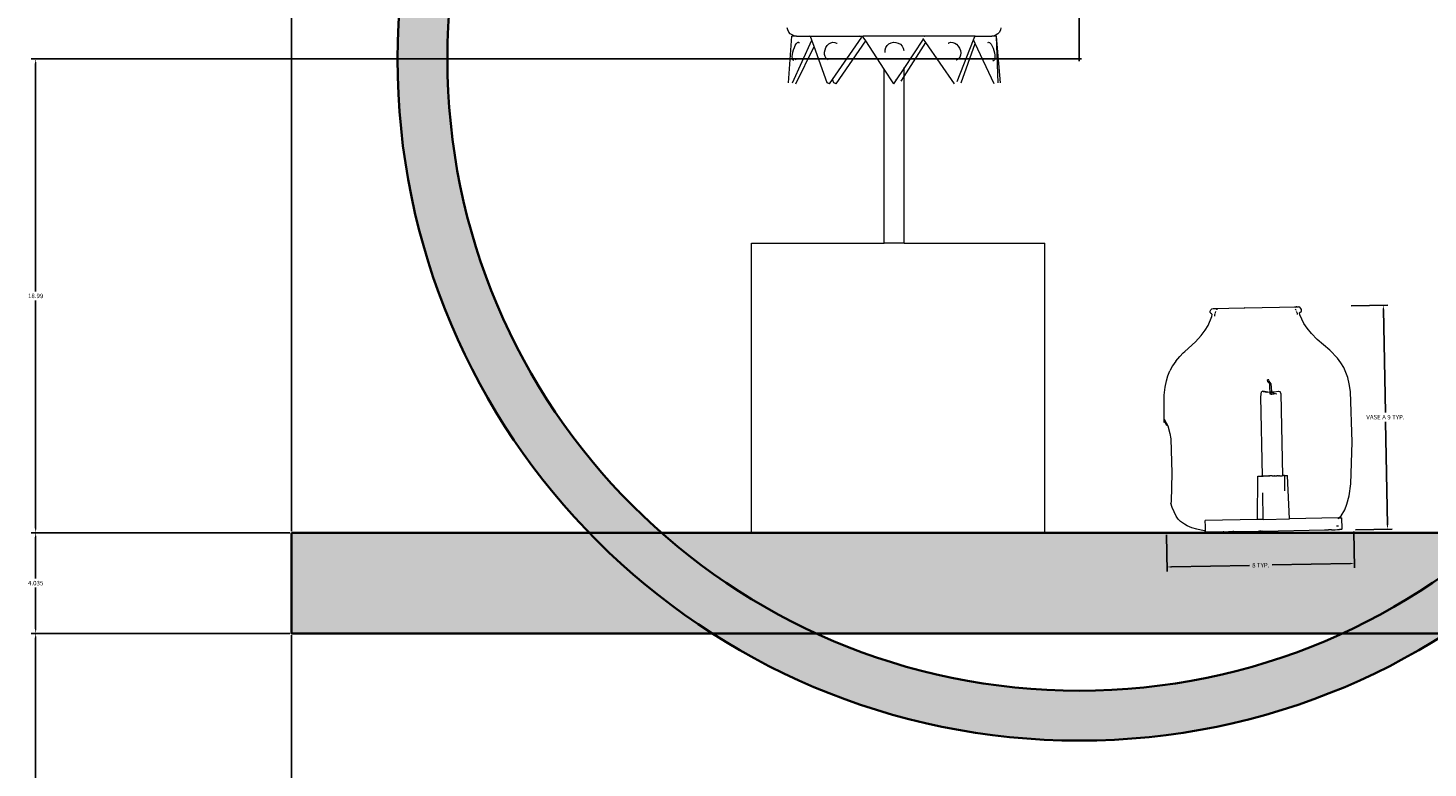
# Model space of a CAD drawing. Units: millimetres. Extents: x 446512 to 447461, y 70395 to 70610.
# Tile 29 of 39: x 447244 to 447300, y 70447 to 70477. Entities that reach past the tile are written whole.
import ezdxf

# ---------------------------------------------------------------- set-up
doc = ezdxf.new("R2010")
doc.units = ezdxf.units.MM
for name, color, linetype, lineweight in [('A-ANNO-DIMS', 2, 'Continuous', 18), ('A-FURN', 7, 'Continuous', 35), ('A-FURN-DECO', 8, 'Continuous', 13), ('A-FURN-PATT', 38, 'Continuous', 13)]:
    doc.layers.add(name, color=color, linetype=linetype, lineweight=lineweight)
doc.styles.get("Standard").update_dxf_attribs({"font": 'arial.ttf'})
doc.dimstyles.get("Standard").update_dxf_attribs({"dimtxt": 0.18, "dimasz": 0.18, "dimexe": 0.18, "dimexo": 0.0625, "dimgap": 0.09, "dimtad": 0, "dimtih": 1, "dimtoh": 1, "dimdec": 4, "dimzin": 0, "dimdsep": 46, "dimtxsty": 'Standard', "dimcen": 0.09, "dimadec": 0, "dimazin": 0, "dimtfac": 1, "dimtdec": 4, "dimtofl": 0, "dimtmove": 0, "dimatfit": 3, "dimfxl": 1, "dimtolj": 1, "dimtzin": 0, "dimarcsym": 0})

# ---------------------------------------------------------------- blocks, each defined once
blk = doc.blocks.new('DECO-SCULPTURE-BIRD')
for p, q in [((1.451, 20.152), (1.431, 20.239)), ((9.995, 20.239), (9.975, 20.152)), ((1.492, 20.071), (1.451, 20.152)), ((1.48, 18.035), (1.609, 19.909)), ((1.551, 20.003), (1.492, 20.071)), ((1.625, 19.952), (1.551, 20.003)), ((1.799, 19.909), (1.609, 19.909)), ((1.709, 19.92), (1.625, 19.952)), ((1.648, 18.028), (2.417, 19.746)), ((1.799, 19.909), (1.709, 19.92)), ((1.799, 19.909), (2.323, 19.909)), ((2.323, 19.909), (2.359, 19.909)), ((2.364, 19.896), (2.323, 19.909)), ((2.364, 19.896), (2.359, 19.909)), ((2.359, 19.909), (4.323, 19.909)), ((2.417, 19.746), (2.364, 19.896)), ((2.508, 19.49), (2.417, 19.746)), ((3.245, 18.169), (4.419, 19.866)), ((3.386, 17.993), (4.578, 19.714)), ((4.323, 19.909), (4.479, 19.909)), ((4.419, 19.866), (4.323, 19.909)), ((4.479, 19.866), (4.479, 19.909)), ((6.726, 19.909), (4.479, 19.909)), ((4.578, 19.714), (4.479, 19.866)), ((5.313, 18.586), (4.578, 19.714)), ((6.112, 18.612), (6.893, 19.784)), ((6.112, 18.284), (6.985, 19.65)), ((6.922, 19.907), (6.726, 19.909)), ((6.893, 19.784), (6.878, 19.805)), ((6.985, 19.65), (6.893, 19.784)), ((6.922, 19.907), (6.926, 19.909)), ((6.926, 19.909), (6.936, 19.909)), ((8.957, 19.909), (6.936, 19.909)), ((8.126, 17.993), (6.985, 19.65)), ((8.239, 18.093), (8.898, 19.762)), ((8.898, 19.762), (8.95, 19.895)), ((8.967, 19.615), (8.898, 19.762)), ((8.95, 19.895), (8.999, 19.909)), ((8.95, 19.895), (8.957, 19.909)), ((8.957, 19.909), (8.999, 19.909)), ((8.999, 19.909), (9.627, 19.909)), ((9.716, 19.92), (9.627, 19.909)), ((9.807, 19.907), (9.627, 19.909)), ((9.801, 19.952), (9.716, 19.92)), ((9.874, 20.003), (9.801, 19.952)), ((9.814, 19.909), (9.807, 19.907)), ((9.816, 19.893), (9.814, 19.909)), ((9.974, 18.035), (9.816, 19.893)), ((9.876, 18.035), (9.816, 19.893)), ((9.934, 20.071), (9.874, 20.003)), ((9.975, 20.152), (9.934, 20.071)), ((1.771, 17.993), (2.508, 19.49)), ((3.027, 18.035), (2.508, 19.49)), ((8.405, 18.035), (8.967, 19.615)), ((9.727, 17.993), (8.967, 19.615)), ((5.313, 11.612), (5.313, 18.586)), ((5.7, 17.993), (5.313, 18.586)), ((5.812, 18.161), (6.112, 18.612)), ((6.112, 18.612), (6.112, 18.655)), ((6.112, 18.284), (6.112, 18.612)), ((3.123, 17.993), (3.027, 18.035)), ((3.123, 17.993), (3.245, 18.169)), ((3.299, 18.035), (3.245, 18.169)), ((3.386, 17.993), (3.299, 18.035)), ((5.7, 17.993), (5.812, 18.161)), ((5.812, 18.161), (5.798, 18.182)), ((5.816, 18.155), (5.812, 18.161)), ((5.995, 18.101), (6.112, 18.284)), ((6.112, 11.612), (6.112, 18.284)), ((0, 0), (0, 11.612)), ((0, 11.612), (5.313, 11.612)), ((6.112, 11.612), (5.313, 11.612)), ((6.112, 11.612), (11.751, 11.612)), ((11.751, 0), (11.751, 11.612)), ((0, 0), (11.751, 0))]:
    blk.add_line(p, q)
blk = doc.blocks.new('DECO-VASE-A')
for p, q in [((1.992, 8.962), (2.04, 8.983)), ((2.04, 8.983), (2.147, 8.974)), ((2.04, 8.983), (3.3, 8.983)), ((3.314, 8.982), (3.3, 8.983)), ((3.314, 8.982), (5.399, 8.983)), ((5.308, 8.977), (5.375, 8.979)), ((5.375, 8.979), (5.332, 8.964)), ((5.399, 8.983), (5.375, 8.979)), ((5.403, 8.983), (5.399, 8.983)), ((5.403, 8.983), (5.462, 8.982)), ((5.511, 8.96), (5.462, 8.982)), ((1.832, 8.302), (1.985, 8.655)), ((1.917, 8.815), (1.923, 8.866)), ((1.917, 8.815), (1.931, 8.786)), ((1.923, 8.866), (1.951, 8.922)), ((1.974, 8.762), (1.931, 8.786)), ((1.951, 8.922), (1.992, 8.962)), ((1.996, 8.731), (1.974, 8.762)), ((1.985, 8.655), (1.996, 8.731)), ((2.1, 8.723), (2.091, 8.673)), ((2.115, 8.769), (2.1, 8.723)), ((2.141, 8.848), (2.125, 8.798)), ((2.147, 8.974), (2.186, 8.942)), ((2.186, 8.942), (2.19, 8.923)), ((5.332, 8.964), (5.314, 8.943)), ((5.325, 8.885), (5.351, 8.865)), ((5.351, 8.865), (5.358, 8.847)), ((5.373, 8.802), (5.377, 8.793)), ((5.382, 8.778), (5.4, 8.725)), ((5.4, 8.725), (5.409, 8.672)), ((5.503, 8.731), (5.511, 8.747)), ((5.515, 8.655), (5.503, 8.731)), ((5.56, 8.904), (5.511, 8.96)), ((5.511, 8.747), (5.566, 8.783)), ((5.668, 8.302), (5.515, 8.655)), ((5.576, 8.866), (5.56, 8.904)), ((5.566, 8.783), (5.581, 8.808)), ((5.581, 8.808), (5.576, 8.866)), ((1.315, 7.659), (1.541, 7.898)), ((1.541, 7.898), (1.71, 8.114)), ((1.71, 8.114), (1.832, 8.302)), ((5.789, 8.114), (5.668, 8.302)), ((5.959, 7.898), (5.789, 8.114)), ((6.185, 7.659), (5.959, 7.898)), ((0.874, 7.277), (1.315, 7.659)), ((6.689, 7.222), (6.185, 7.659)), ((0.508, 6.898), (0.375, 6.707)), ((0.508, 6.898), (0.67, 7.084)), ((0.67, 7.084), (0.81, 7.222)), ((0.81, 7.222), (0.874, 7.277)), ((6.991, 6.898), (6.689, 7.222)), ((7.124, 6.707), (6.991, 6.898)), ((0.117, 6.113), (0.182, 6.314)), ((0.182, 6.314), (0.267, 6.512)), ((0.375, 6.707), (0.267, 6.512)), ((7.232, 6.512), (7.124, 6.707)), ((7.317, 6.314), (7.232, 6.512)), ((7.382, 6.113), (7.317, 6.314)), ((0.02, 5.541), (0.06, 5.856)), ((0.06, 5.856), (0.117, 6.113)), ((3.97, 5.625), (3.916, 5.6)), ((4.168, 5.588), (3.97, 5.625)), ((4.129, 5.567), (3.989, 5.611)), ((3.989, 5.611), (4.168, 5.588)), ((4.217, 6.081), (4.173, 6.078)), ((4.184, 5.991), (4.173, 6.078)), ((4.258, 5.909), (4.184, 5.991)), ((4.227, 6.021), (4.217, 6.081)), ((4.297, 5.928), (4.227, 6.021)), ((4.261, 5.759), (4.258, 5.909)), ((4.266, 5.588), (4.261, 5.759)), ((4.297, 5.928), (4.32, 5.588)), ((4.422, 5.588), (4.602, 5.615)), ((4.602, 5.615), (4.675, 5.587)), ((7.44, 5.856), (7.382, 6.113)), ((7.479, 5.541), (7.44, 5.856)), ((0.002, 4.579), (0.02, 5.541)), ((3.893, 5.401), (3.916, 5.6)), ((3.893, 2.225), (3.893, 5.401)), ((4.168, 5.588), (4.266, 5.588)), ((4.267, 5.562), (4.168, 5.588)), ((4.268, 5.524), (4.24, 5.533)), ((4.267, 5.562), (4.266, 5.588)), ((4.266, 5.588), (4.32, 5.588)), ((4.322, 5.548), (4.267, 5.562)), ((4.267, 5.554), (4.267, 5.559)), ((4.268, 5.524), (4.267, 5.541)), ((4.295, 5.515), (4.268, 5.524)), ((4.268, 5.504), (4.268, 5.524)), ((4.303, 5.503), (4.268, 5.504)), ((4.295, 5.515), (4.325, 5.513)), ((4.303, 5.503), (4.325, 5.502)), ((4.32, 5.588), (4.322, 5.548)), ((4.32, 5.588), (4.422, 5.588)), ((4.525, 5.496), (4.322, 5.548)), ((4.323, 5.541), (4.324, 5.523)), ((4.325, 5.513), (4.325, 5.502)), ((4.325, 5.513), (4.428, 5.504)), ((4.691, 5.523), (4.675, 5.587)), ((4.691, 5.523), (4.695, 2.225)), ((7.516, 3.52), (7.479, 5.541)), ((0, 4.513), (0.002, 4.579)), ((0.002, 4.51), (0, 4.513)), ((0, 4.439), (0.002, 4.51)), ((0.002, 4.579), (0.134, 4.312)), ((0.052, 4.428), (0.002, 4.51)), ((0.095, 4.312), (0.052, 4.428)), ((0.134, 4.312), (0.217, 3.999)), ((0.217, 3.999), (0.244, 3.785)), ((0.244, 3.785), (0.269, 2.409)), ((7.431, 1.848), (7.516, 3.52)), ((0.269, 2.409), (0.211, 1.27)), ((3.665, 0.487), (3.705, 2.219)), ((3.705, 2.219), (3.712, 2.225)), ((3.712, 2.225), (3.763, 2.225)), ((3.763, 2.225), (3.766, 2.225)), ((3.766, 2.225), (3.789, 2.225)), ((3.789, 2.225), (3.795, 2.225)), ((3.795, 2.225), (3.797, 2.225)), ((3.797, 2.225), (3.813, 2.225)), ((3.813, 2.225), (3.821, 2.225)), ((3.821, 2.225), (3.825, 2.225)), ((3.825, 2.225), (3.828, 2.225)), ((3.828, 2.225), (3.832, 2.225)), ((3.832, 2.225), (3.838, 2.225)), ((3.842, 2.225), (3.838, 2.225)), ((3.838, 2.225), (3.838, 2.219)), ((3.842, 2.225), (3.844, 2.225)), ((3.844, 2.225), (3.852, 2.225)), ((3.864, 2.225), (3.852, 2.225)), ((3.867, 2.225), (3.864, 2.225)), ((3.867, 2.225), (3.878, 2.225)), ((3.878, 2.225), (3.881, 2.225)), ((3.881, 2.225), (3.883, 2.225)), ((3.883, 2.225), (3.893, 2.225)), ((3.893, 2.219), (3.893, 2.225)), ((3.908, 2.225), (3.893, 2.225)), ((3.908, 2.225), (3.927, 2.225)), ((3.992, 2.225), (3.927, 2.225)), ((4.002, 2.225), (3.992, 2.225)), ((4.002, 2.225), (4.053, 2.225)), ((4.053, 2.225), (4.065, 2.225)), ((4.065, 2.225), (4.148, 2.225)), ((4.163, 2.225), (4.148, 2.225)), ((4.163, 2.225), (4.192, 2.225)), ((4.278, 2.225), (4.192, 2.225)), ((4.278, 2.225), (4.283, 2.225)), ((4.283, 2.225), (4.374, 2.225)), ((4.394, 2.225), (4.374, 2.225)), ((4.394, 2.225), (4.451, 2.225)), ((4.451, 2.225), (4.462, 2.225)), ((4.496, 2.225), (4.462, 2.225)), ((4.5, 2.225), (4.496, 2.225)), ((4.505, 2.225), (4.5, 2.225)), ((4.505, 2.225), (4.508, 2.225)), ((4.508, 2.225), (4.511, 2.225)), ((4.511, 2.225), (4.541, 2.225)), ((4.553, 2.225), (4.541, 2.225)), ((4.578, 2.225), (4.553, 2.225)), ((4.578, 2.225), (4.583, 2.225)), ((4.583, 2.225), (4.65, 2.225)), ((4.659, 2.225), (4.65, 2.225)), ((4.659, 2.225), (4.683, 2.225)), ((4.69, 2.225), (4.683, 2.225)), ((4.695, 2.225), (4.69, 2.225)), ((4.695, 2.225), (4.695, 2.219)), ((4.697, 2.225), (4.695, 2.225)), ((4.702, 2.225), (4.697, 2.225)), ((4.704, 2.225), (4.702, 2.225)), ((4.704, 2.225), (4.718, 2.225)), ((4.722, 2.225), (4.718, 2.225)), ((4.74, 2.225), (4.722, 2.225)), ((4.744, 2.225), (4.74, 2.225)), ((4.744, 2.225), (4.756, 2.225)), ((4.769, 2.225), (4.756, 2.225)), ((4.769, 2.225), (4.76, 1.611)), ((4.773, 2.225), (4.769, 2.225)), ((4.777, 2.225), (4.773, 2.225)), ((4.777, 2.225), (4.802, 2.225)), ((4.802, 2.225), (4.807, 2.225)), ((4.807, 2.225), (4.813, 2.225)), ((4.813, 2.225), (4.834, 2.225)), ((4.834, 2.225), (4.837, 2.225)), ((4.837, 2.225), (4.84, 2.225)), ((4.84, 2.225), (4.849, 2.225)), ((4.849, 2.225), (4.895, 2.225)), ((4.902, 2.219), (4.895, 2.225)), ((4.942, 0.487), (4.902, 2.219)), ((7.347, 1.371), (7.431, 1.848)), ((0.211, 1.27), (0.2, 1.204)), ((0.248, 1.032), (0.2, 1.204)), ((3.893, 0.487), (3.893, 1.548)), ((7.251, 1.032), (7.347, 1.371)), ((0.41, 0.681), (0.248, 1.032)), ((0.488, 0.567), (0.41, 0.681)), ((0.576, 0.472), (0.488, 0.567)), ((6.926, 0.487), (7.011, 0.567)), ((7.011, 0.567), (7.16, 0.81)), ((7.16, 0.81), (7.251, 1.032)), ((0.727, 0.355), (0.576, 0.472)), ((0.839, 0.288), (0.727, 0.355)), ((1.025, 0.205), (0.839, 0.288)), ((1.227, 0.14), (1.025, 0.205)), ((1.518, 0.077), (1.227, 0.14)), ((1.567, 0.071), (1.518, 0.077)), ((1.567, 0.24), (1.568, 0.487)), ((1.567, 0.071), (1.567, 0.24)), ((1.567, 0.045), (1.567, 0.071)), ((1.588, 0.02), (1.567, 0.045)), ((3.665, 0.487), (1.568, 0.487)), ((2.274, 0.02), (1.588, 0.02)), ((2.295, 0.021), (2.274, 0.02)), ((2.306, 0.02), (2.295, 0.021)), ((2.306, 0.02), (2.665, 0.02)), ((2.665, 0.02), (2.495, 0.021)), ((2.684, 0.022), (2.665, 0.02)), ((2.704, 0.02), (2.684, 0.022)), ((2.704, 0.02), (3.676, 0.02)), ((3.521, 0), (3.685, 0.017)), ((3.521, 0), (3.97, 0)), ((3.893, 0.487), (3.665, 0.487)), ((3.685, 0.017), (3.676, 0.02)), ((3.685, 0.017), (3.729, 0.02)), ((3.775, 0.017), (3.729, 0.02)), ((3.793, 0.02), (3.775, 0.017)), ((3.793, 0.02), (3.84, 0.017)), ((3.84, 0.017), (3.859, 0.02)), ((3.97, 0), (3.84, 0.017)), ((3.859, 0.02), (6.333, 0.02)), ((3.893, 0.487), (4.942, 0.487)), ((6.889, 0.487), (4.942, 0.487)), ((6.333, 0.02), (6.501, 0.021)), ((6.622, 0.02), (6.501, 0.021)), ((6.622, 0.02), (6.643, 0.02)), ((6.643, 0.02), (6.645, 0.02)), ((6.643, 0.02), (6.647, 0.02)), ((6.647, 0.02), (6.749, 0.02)), ((6.749, 0.02), (6.768, 0.02)), ((6.768, 0.02), (6.77, 0.02)), ((6.77, 0.02), (6.854, 0.02)), ((6.854, 0.02), (6.911, 0.02)), ((6.889, 0.452), (6.926, 0.487)), ((6.889, 0.487), (6.926, 0.487)), ((6.911, 0.02), (6.933, 0.02)), ((6.938, 0.487), (6.926, 0.487)), ((6.945, 0.02), (6.933, 0.02)), ((6.953, 0.487), (6.938, 0.487)), ((7.019, 0.02), (6.945, 0.02)), ((6.953, 0.487), (7.039, 0.487)), ((7.019, 0.02), (7.039, 0.045)), ((7.039, 0.045), (7.039, 0.487))]:
    blk.add_line(p, q)
blk = doc.blocks.new('*D7')
at = {"layer": 'A-ANNO-DIMS', "color": 0, "lineweight": -2, "transparency": 16777216}
for p, q in [((447297.404, 70465.99), (447298.869, 70466.018)), ((447298.692, 70465.834), (447298.77, 70461.707)), ((447298.855, 70457.214), (447298.777, 70461.341)), ((447297.574, 70457.009), (447299.039, 70457.037))]:
    blk.add_line(p, q, dxfattribs=at)
at = {"layer": 'A-ANNO-DIMS', "color": 0, "transparency": 16777216}
for points in [[(447298.722, 70465.835), (447298.662, 70465.834), (447298.689, 70466.014)], [(447298.885, 70457.214), (447298.825, 70457.213), (447298.859, 70457.034)]]:
    blk.add_solid(points, dxfattribs=at)
at = {"layer": 'Defpoints', "color": 0, "transparency": 16777216}
for p in [(447297.342, 70465.989), (447298.689, 70466.014), (447297.512, 70457.008)]:
    blk.add_point(p, dxfattribs=at)
at = {"layer": 'A-ANNO-DIMS', "color": 0, "transparency": 16777216, "insert": (447298.774, 70461.524), "char_height": 0.18, "attachment_point": 5}
blk.add_mtext('\\A1;VASE A 9 TYP.', dxfattribs=at)
blk = doc.blocks.new('*D8')
at = {"layer": 'A-ANNO-DIMS', "color": 0, "lineweight": -2, "transparency": 16777216}
for p, q in [((447289.998, 70456.803), (447290.026, 70455.339)), ((447297.513, 70456.946), (447297.54, 70455.481)), ((447297.357, 70455.658), (447294.238, 70455.599)), ((447290.202, 70455.522), (447293.321, 70455.581))]:
    blk.add_line(p, q, dxfattribs=at)
at = {"layer": 'A-ANNO-DIMS', "color": 0, "transparency": 16777216}
for points in [[(447297.357, 70455.688), (447297.358, 70455.628), (447297.537, 70455.661)], [(447290.202, 70455.552), (447290.203, 70455.492), (447290.022, 70455.519)]]:
    blk.add_solid(points, dxfattribs=at)
at = {"layer": 'Defpoints', "color": 0, "transparency": 16777216}
for p in [(447289.997, 70456.866), (447297.512, 70457.008), (447297.537, 70455.661)]:
    blk.add_point(p, dxfattribs=at)
at = {"layer": 'A-ANNO-DIMS', "color": 0, "transparency": 16777216, "insert": (447293.78, 70455.59), "char_height": 0.18, "attachment_point": 5}
blk.add_mtext('\\A1;8 TYP.', dxfattribs=at)
blk = doc.blocks.new('*D61')
at = {"layer": 'A-ANNO-DIMS', "color": 0, "lineweight": -2, "transparency": 16777216}
for p, q in [((447254.943, 70452.792), (447254.943, 70394.885)), ((447450.532, 70432.19), (447450.532, 70394.885)), ((447255.123, 70395.065), (447352.352, 70395.065)), ((447450.352, 70395.065), (447353.122, 70395.065))]:
    blk.add_line(p, q, dxfattribs=at)
at = {"layer": 'A-ANNO-DIMS', "color": 0, "transparency": 16777216}
for points in [[(447255.123, 70395.095), (447255.123, 70395.035), (447254.943, 70395.065)], [(447450.352, 70395.095), (447450.352, 70395.035), (447450.532, 70395.065)]]:
    blk.add_solid(points, dxfattribs=at)
at = {"layer": 'Defpoints', "color": 0, "transparency": 16777216}
for p in [(447254.943, 70452.855), (447450.532, 70432.253), (447450.532, 70395.065)]:
    blk.add_point(p, dxfattribs=at)
at = {"layer": 'A-ANNO-DIMS', "color": 0, "transparency": 16777216, "insert": (447352.737, 70395.065), "char_height": 0.18, "attachment_point": 5}
blk.add_mtext('\\A1;195.6', dxfattribs=at)
blk = doc.blocks.new('*D62')
at = {"layer": 'A-ANNO-DIMS', "color": 0, "lineweight": -2, "transparency": 16777216}
for p, q in [((447254.943, 70456.952), (447254.943, 70610.145)), ((447255.123, 70609.965), (447270.262, 70609.965)), ((447286.329, 70609.965), (447271.189, 70609.965)), ((447286.509, 70475.943), (447286.509, 70610.145))]:
    blk.add_line(p, q, dxfattribs=at)
at = {"layer": 'A-ANNO-DIMS', "color": 0, "transparency": 16777216}
for points in [[(447255.123, 70609.995), (447255.123, 70609.935), (447254.943, 70609.965)], [(447286.329, 70609.995), (447286.329, 70609.935), (447286.509, 70609.965)]]:
    blk.add_solid(points, dxfattribs=at)
at = {"layer": 'Defpoints', "color": 0, "transparency": 16777216}
for p in [(447286.509, 70609.965), (447286.509, 70475.881), (447254.943, 70456.89)]:
    blk.add_point(p, dxfattribs=at)
at = {"layer": 'A-ANNO-DIMS', "color": 0, "transparency": 16777216, "insert": (447270.726, 70609.965), "char_height": 0.18, "attachment_point": 5}
blk.add_mtext('\\A1;31.566', dxfattribs=at)
blk = doc.blocks.new('*D63')
at = {"layer": 'A-ANNO-DIMS', "color": 0, "lineweight": -2, "transparency": 16777216}
for p, q in [((447286.509, 70475.943), (447286.509, 70610.145)), ((447286.689, 70609.965), (447312.886, 70609.965)), ((447339.869, 70609.965), (447313.672, 70609.965)), ((447340.049, 70506.612), (447340.049, 70610.145))]:
    blk.add_line(p, q, dxfattribs=at)
at = {"layer": 'A-ANNO-DIMS', "color": 0, "transparency": 16777216}
for points in [[(447286.689, 70609.995), (447286.689, 70609.935), (447286.509, 70609.965)], [(447339.869, 70609.995), (447339.869, 70609.935), (447340.049, 70609.965)]]:
    blk.add_solid(points, dxfattribs=at)
at = {"layer": 'Defpoints', "color": 0, "transparency": 16777216}
for p in [(447340.049, 70609.965), (447340.049, 70506.55), (447286.509, 70475.881)]:
    blk.add_point(p, dxfattribs=at)
at = {"layer": 'A-ANNO-DIMS', "color": 0, "transparency": 16777216, "insert": (447313.279, 70609.965), "char_height": 0.18, "attachment_point": 5}
blk.add_mtext('\\A1;53.54', dxfattribs=at)
blk = doc.blocks.new('*D72')
at = {"layer": 'A-ANNO-DIMS', "color": 0, "lineweight": -2, "transparency": 16777216}
for p, q in [((447254.88, 70452.855), (447244.513, 70452.855)), ((447244.693, 70452.675), (447244.693, 70429.266)), ((447244.693, 70405.495), (447244.693, 70428.903)), ((447365.363, 70405.315), (447244.513, 70405.315))]:
    blk.add_line(p, q, dxfattribs=at)
at = {"layer": 'A-ANNO-DIMS', "color": 0, "transparency": 16777216}
for points in [[(447244.663, 70452.675), (447244.723, 70452.675), (447244.693, 70452.855)], [(447244.663, 70405.495), (447244.723, 70405.495), (447244.693, 70405.315)]]:
    blk.add_solid(points, dxfattribs=at)
at = {"layer": 'Defpoints', "color": 0, "transparency": 16777216}
for p in [(447244.693, 70452.855), (447254.943, 70452.855), (447365.425, 70405.315)]:
    blk.add_point(p, dxfattribs=at)
at = {"layer": 'A-ANNO-DIMS', "color": 0, "transparency": 16777216, "insert": (447244.693, 70429.085), "char_height": 0.18, "attachment_point": 5}
blk.add_mtext('\\A1;47.54', dxfattribs=at)
blk = doc.blocks.new('*D73')
at = {"layer": 'A-ANNO-DIMS', "color": 0, "lineweight": -2, "transparency": 16777216}
for p, q in [((447254.88, 70456.89), (447244.513, 70456.89)), ((447244.693, 70456.71), (447244.693, 70455.054)), ((447244.693, 70453.035), (447244.693, 70454.691)), ((447254.88, 70452.855), (447244.513, 70452.855))]:
    blk.add_line(p, q, dxfattribs=at)
at = {"layer": 'A-ANNO-DIMS', "color": 0, "transparency": 16777216}
for points in [[(447244.663, 70456.71), (447244.723, 70456.71), (447244.693, 70456.89)], [(447244.663, 70453.035), (447244.723, 70453.035), (447244.693, 70452.855)]]:
    blk.add_solid(points, dxfattribs=at)
at = {"layer": 'Defpoints', "color": 0, "transparency": 16777216}
for p in [(447244.693, 70456.89), (447254.943, 70456.89), (447254.943, 70452.855)]:
    blk.add_point(p, dxfattribs=at)
at = {"layer": 'A-ANNO-DIMS', "color": 0, "transparency": 16777216, "insert": (447244.693, 70454.872), "char_height": 0.18, "attachment_point": 5}
blk.add_mtext('\\A1;4.035', dxfattribs=at)
blk = doc.blocks.new('*D74')
at = {"layer": 'A-ANNO-DIMS', "color": 0, "lineweight": -2, "transparency": 16777216}
for p, q in [((447286.446, 70475.881), (447244.513, 70475.881)), ((447244.693, 70475.701), (447244.693, 70466.567)), ((447244.693, 70457.07), (447244.693, 70466.203)), ((447254.88, 70456.89), (447244.513, 70456.89))]:
    blk.add_line(p, q, dxfattribs=at)
at = {"layer": 'A-ANNO-DIMS', "color": 0, "transparency": 16777216}
for points in [[(447244.663, 70475.701), (447244.723, 70475.701), (447244.693, 70475.881)], [(447244.663, 70457.07), (447244.723, 70457.07), (447244.693, 70456.89)]]:
    blk.add_solid(points, dxfattribs=at)
at = {"layer": 'Defpoints', "color": 0, "transparency": 16777216}
for p in [(447244.693, 70475.881), (447286.509, 70475.881), (447254.943, 70456.89)]:
    blk.add_point(p, dxfattribs=at)
at = {"layer": 'A-ANNO-DIMS', "color": 0, "transparency": 16777216, "insert": (447244.693, 70466.385), "char_height": 0.18, "attachment_point": 5}
blk.add_mtext('\\A1;18.99', dxfattribs=at)
blk = doc.blocks.new('*D79')
at = {"layer": 'A-ANNO-DIMS', "color": 0, "lineweight": -2, "transparency": 16777216}
for p, q in [((447286.419, 70475.881), (447286.599, 70475.881)), ((447286.509, 70475.791), (447286.509, 70475.971)), ((447330.218, 70475.881), (447314.007, 70475.881))]:
    blk.add_line(p, q, dxfattribs=at)
at = {"layer": 'A-ANNO-DIMS', "color": 0, "transparency": 16777216}
blk.add_solid([(447314.007, 70475.911), (447314.007, 70475.851), (447313.827, 70475.881)], dxfattribs=at)
at = {"layer": 'Defpoints', "color": 0, "transparency": 16777216}
for p in [(447259.19, 70475.88), (447313.827, 70475.881)]:
    blk.add_point(p, dxfattribs=at)
at = {"layer": 'A-ANNO-DIMS', "color": 0, "transparency": 16777216, "insert": (447330.709, 70475.881), "char_height": 0.18, "attachment_point": 5}
blk.add_mtext('\\A1;∅54.64', dxfattribs=at)
blk = doc.blocks.new('*D80')
at = {"layer": 'A-ANNO-DIMS', "color": 0, "lineweight": -2, "transparency": 16777216}
for p, q in [((447286.419, 70475.881), (447286.599, 70475.881)), ((447286.509, 70475.791), (447286.509, 70475.971)), ((447327.018, 70475.881), (447312.007, 70475.881))]:
    blk.add_line(p, q, dxfattribs=at)
at = {"layer": 'A-ANNO-DIMS', "color": 0, "transparency": 16777216}
blk.add_solid([(447312.007, 70475.911), (447312.007, 70475.851), (447311.827, 70475.881)], dxfattribs=at)
at = {"layer": 'Defpoints', "color": 0, "transparency": 16777216}
for p in [(447261.19, 70475.88), (447311.827, 70475.881)]:
    blk.add_point(p, dxfattribs=at)
at = {"layer": 'A-ANNO-DIMS', "color": 0, "transparency": 16777216, "insert": (447327.509, 70475.881), "char_height": 0.18, "attachment_point": 5}
blk.add_mtext('\\A1;∅50.64', dxfattribs=at)

msp = doc.modelspace()

# ---------------------------------------------------------------- hatches: boundary and pattern name
at = {"layer": 'A-FURN-PATT'}
h = msp.add_hatch(color=256, dxfattribs=at)
h.dxf.hatch_style = 1
h.paths.add_polyline_path([(447259.1901, 70475.8806, 0.1945594), (447266.8704, 70456.89), (447269.7639, 70456.89, -0.2152771), (447261.1901, 70475.8806, -1), (447311.827, 70475.8806, -0.2152771), (447303.2532, 70456.89), (447306.1467, 70456.89, 0.1945594), (447313.827, 70475.8806, 1)])
h.paths.add_polyline_path([(447301.2097, 70452.855), (447297.037, 70452.855, -0.2177821), (447275.9801, 70452.855), (447271.8074, 70452.855, 0.2920128)])
h.paths.add_polyline_path([(447269.7639, 70456.89), (447266.8704, 70456.89, 0.0585505), (447271.8074, 70452.855), (447275.9801, 70452.855, -0.0735735)])
h.paths.add_polyline_path([(447306.1467, 70456.89), (447303.2532, 70456.89, -0.0735735), (447297.037, 70452.855), (447301.2097, 70452.855, 0.0585505)])
h = msp.add_hatch(color=256, dxfattribs=at)
h.dxf.hatch_style = 1
h.paths.add_polyline_path([(447280.3184, 70456.89), (447254.9427, 70456.89), (447254.9427, 70452.855), (447280.3184, 70452.855)])
h.paths.add_polyline_path([(447365.4251, 70456.89), (447340.9075, 70456.89), (447340.9075, 70452.855), (447365.4251, 70452.855)])
h.paths.add_polyline_path([(447340.9075, 70456.89), (447280.3184, 70456.89), (447280.3184, 70452.855), (447340.9075, 70452.855)])

# ---------------------------------------------------------------- linework, layer by layer
at = {"layer": 'A-FURN'}
msp.add_lwpolyline([(447254.9427, 70456.89), (447365.4251, 70456.89), (447365.4251, 70452.855), (447254.9427, 70452.855)], close=True, dxfattribs=at)
for radius in [27.3185, 25.3185]:
    msp.add_circle((447286.5086, 70475.8806), radius, dxfattribs=at)
at = {"layer": 'A-FURN-DECO'}
for p, q in [((447275.0904, 70476.3352), (447275.1259, 70476.416)), ((447275.1259, 70476.416), (447275.1631, 70476.4811)), ((447275.1631, 70476.4811), (447275.1995, 70476.5262)), ((447275.1995, 70476.5262), (447275.2326, 70476.5481)), ((447275.2326, 70476.5481), (447275.2601, 70476.5455)), ((447275.2652, 70476.539), (447275.2601, 70476.5455)), ((447275.2652, 70476.539), (447275.2927, 70476.5363)), ((447276.3564, 70476.3352), (447276.4104, 70476.416)), ((447276.4104, 70476.416), (447276.4778, 70476.4811)), ((447276.4778, 70476.4811), (447276.5538, 70476.5262)), ((447276.5538, 70476.5262), (447276.6333, 70476.5481)), ((447276.6333, 70476.5481), (447276.7109, 70476.5455)), ((447276.7109, 70476.5455), (447276.7839, 70476.5162)), ((447276.7839, 70476.5162), (447276.802, 70476.5092)), ((447278.7581, 70476.3352), (447278.8096, 70476.416)), ((447278.8096, 70476.416), (447278.8809, 70476.4811)), ((447278.8809, 70476.4811), (447278.9673, 70476.5262)), ((447278.9673, 70476.5262), (447279.0628, 70476.5481)), ((447279.0628, 70476.5481), (447279.1609, 70476.5455)), ((447279.1609, 70476.5455), (447279.255, 70476.5184)), ((447279.255, 70476.5184), (447279.3386, 70476.4687)), ((447279.3386, 70476.4687), (447279.406, 70476.3998)), ((447279.406, 70476.3998), (447279.4527, 70476.3163)), ((447281.2599, 70476.517), (447281.2708, 70476.5203)), ((447281.2708, 70476.5203), (447281.2792, 70476.5262)), ((447281.2792, 70476.5262), (447281.3544, 70476.5481)), ((447281.3544, 70476.5481), (447281.4355, 70476.5455)), ((447281.4355, 70476.5455), (447281.517, 70476.5184)), ((447281.517, 70476.5184), (447281.5933, 70476.4687)), ((447281.5933, 70476.4687), (447281.6592, 70476.3998)), ((447281.6592, 70476.3998), (447281.7103, 70476.3163)), ((447282.8393, 70476.539), (447282.8715, 70476.5481)), ((447282.8393, 70476.539), (447282.8588, 70476.5374)), ((447282.8715, 70476.5481), (447282.9046, 70476.5455)), ((447282.9046, 70476.5455), (447282.9425, 70476.5184)), ((447282.9425, 70476.5184), (447282.9827, 70476.4687)), ((447282.9827, 70476.4687), (447283.0224, 70476.3998)), ((447283.0224, 70476.3998), (447283.059, 70476.3163)), ((447275.0087, 70475.9739), (447275.0167, 70476.0573)), ((447275.0104, 70475.905), (447275.0087, 70475.9739)), ((447275.0217, 70475.8553), (447275.0104, 70475.905)), ((447275.0167, 70476.0573), (447275.0339, 70476.1496)), ((447275.0418, 70475.8282), (447275.0217, 70475.8553)), ((447275.0339, 70476.1496), (447275.059, 70476.2443)), ((447275.059, 70476.2443), (447275.0904, 70476.3352)), ((447275.1221, 70475.8719), (447275.1336, 70475.8475)), ((447275.1336, 70475.8475), (447275.1391, 70475.8435)), ((447275.1417, 70475.8977), (447275.144, 70475.8834)), ((447276.3017, 70476.1496), (447276.3193, 70476.2443)), ((447276.3048, 70476.0573), (447276.3017, 70476.1496)), ((447276.3284, 70475.9739), (447276.3048, 70476.0573)), ((447276.3193, 70476.2443), (447276.3564, 70476.3352)), ((447276.3709, 70475.905), (447276.3284, 70475.9739)), ((447276.4293, 70475.8553), (447276.3709, 70475.905)), ((447276.4499, 70475.8462), (447276.4293, 70475.8553)), ((447278.7273, 70476.1404), (447278.7276, 70476.1486)), ((447278.7276, 70476.1486), (447278.7301, 70476.2443)), ((447278.7301, 70476.2443), (447278.7581, 70476.3352)), ((447279.4527, 70476.3163), (447279.4754, 70476.2241)), ((447279.4754, 70476.215), (447279.4754, 70476.2241)), ((447281.5923, 70475.8443), (447281.5839, 70475.8384)), ((447281.5923, 70475.8443), (447281.6032, 70475.8475)), ((447281.6674, 70475.8926), (447281.6032, 70475.8475)), ((447281.7161, 70475.9577), (447281.6674, 70475.8926)), ((447281.7103, 70476.3163), (447281.7431, 70476.2241)), ((447281.7461, 70476.0385), (447281.7161, 70475.9577)), ((447281.7431, 70476.2241), (447281.7553, 70476.1293)), ((447281.7553, 70476.1293), (447281.7461, 70476.0385)), ((447283.059, 70476.3163), (447283.0898, 70476.2241)), ((447283.1057, 70475.8475), (447283.0797, 70475.8255)), ((447283.0898, 70476.2241), (447283.1129, 70476.1293)), ((447283.1229, 70475.8926), (447283.1057, 70475.8475)), ((447283.1129, 70476.1293), (447283.1266, 70476.0385)), ((447283.13, 70475.9577), (447283.1229, 70475.8926)), ((447283.1266, 70476.0385), (447283.13, 70475.9577)), ((447275.0695, 70475.8257), (447275.0418, 70475.8282)), ((447275.0744, 70475.8191), (447275.0695, 70475.8257)), ((447283.0602, 70475.8271), (447283.0476, 70475.8164)), ((447283.0476, 70475.8164), (447283.0797, 70475.8255)), ((447296.8656, 70457.1508), (447296.8144, 70457.1504)), ((447296.8901, 70457.1508), (447296.8656, 70457.1508))]:
    msp.add_line(p, q, dxfattribs=at)

# ---------------------------------------------------------------- block references
msp.add_blockref('DECO-SCULPTURE-BIRD', (447273.375, 70456.89), dxfattribs=at)
at = {"layer": 'A-FURN-DECO', "rotation": 1.084701014404241}
msp.add_blockref('DECO-VASE-A', (447289.9969, 70456.8657), dxfattribs=at)

# ---------------------------------------------------------------- dimensions: what is measured, and where the dimension line sits
at = {"layer": 'A-ANNO-DIMS'}
for base, p1, p2, override, picture, middle in [((447286.5086, 70609.9647), (447254.9427, 70456.89), (447286.5086, 70475.8806), {"dimdec": 3, "dimlfac": 1, "dimrnd": 0, "dimzin": 0, "dimdsep": 46, "dimlunit": 2}, '*D62', (447270.7256, 70609.9647)), ((447340.0494, 70609.9647), (447286.5086, 70475.8806), (447340.0494, 70506.5496), {"dimdec": 2, "dimlfac": 1, "dimrnd": 0, "dimzin": 0, "dimdsep": 46, "dimlunit": 2}, '*D63', (447313.279, 70609.9647)), ((447450.5318, 70395.0645), (447254.9427, 70452.855), (447450.5318, 70432.2526), {"dimdec": 1, "dimlfac": 1, "dimrnd": 0, "dimzin": 0, "dimdsep": 46, "dimlunit": 2}, '*D61', (447352.7372, 70395.0645))]:
    dim = msp.add_linear_dim(base=base, p1=p1, p2=p2, dimstyle='Standard', override=override, dxfattribs=at)
    dim.commit()
    dim.dimension.update_dxf_attribs({"geometry": picture, "text_midpoint": middle})
for base, p1, p2, override, picture, middle in [((447244.6927, 70475.8806), (447254.9427, 70456.89), (447286.5086, 70475.8806), {"dimdec": 2, "dimlfac": 1, "dimrnd": 0, "dimzin": 0, "dimdsep": 46, "dimlunit": 2}, '*D74', (447244.6927, 70466.3853)), ((447244.6927, 70456.89), (447254.9427, 70452.855), (447254.9427, 70456.89), {"dimdec": 3, "dimlfac": 1, "dimrnd": 0, "dimzin": 0, "dimdsep": 46, "dimlunit": 2}, '*D73', (447244.6927, 70454.8725)), ((447244.6927, 70452.855), (447365.4251, 70405.3145), (447254.9427, 70452.855), {"dimdec": 2, "dimlfac": 1, "dimrnd": 0, "dimzin": 0, "dimdsep": 46, "dimlunit": 2}, '*D72', (447244.6927, 70429.0848))]:
    dim = msp.add_linear_dim(base=base, p1=p1, p2=p2, angle=90, dimstyle='Standard', override=override, dxfattribs=at)
    dim.commit()
    dim.dimension.update_dxf_attribs({"geometry": picture, "text_midpoint": middle})
for p1, p2, picture, middle in [((447259.1901, 70475.8801), (447313.827, 70475.881), '*D79', (447330.2181, 70475.8813)), ((447261.1901, 70475.8801), (447311.827, 70475.881), '*D80', (447327.0181, 70475.8813))]:
    dim = msp.add_diameter_dim_2p(p1=p1, p2=p2, dimstyle='Standard', override={"dimdec": 2, "dimlfac": 1, "dimrnd": 0, "dimzin": 0, "dimdsep": 46, "dimlunit": 2}, dxfattribs=at)
    dim.commit()
    dim.dimension.update_dxf_attribs({"geometry": picture, "text_midpoint": middle, "dimtype": 163})
for base, p1, p2, angle, text, picture, middle in [((447298.6886, 70466.0144), (447297.5116, 70457.0081), (447297.3415, 70465.9889), 91.0847, 'VASE A <> TYP.', '*D7', (447298.7737, 70461.524)), ((447297.5371, 70455.661), (447289.9967, 70456.8659), (447297.5116, 70457.0081), 1.0847, '<> TYP.', '*D8', (447293.7797, 70455.5899))]:
    dim = msp.add_linear_dim(base=base, p1=p1, p2=p2, angle=angle, text=text, dimstyle='Standard', override={"dimdec": 0, "dimlfac": 1, "dimrnd": 0, "dimzin": 0, "dimdsep": 46, "dimlunit": 2}, dxfattribs=at)
    dim.commit()
    dim.dimension.update_dxf_attribs({"geometry": picture, "text_midpoint": middle})

doc.saveas('drawing.dxf')
